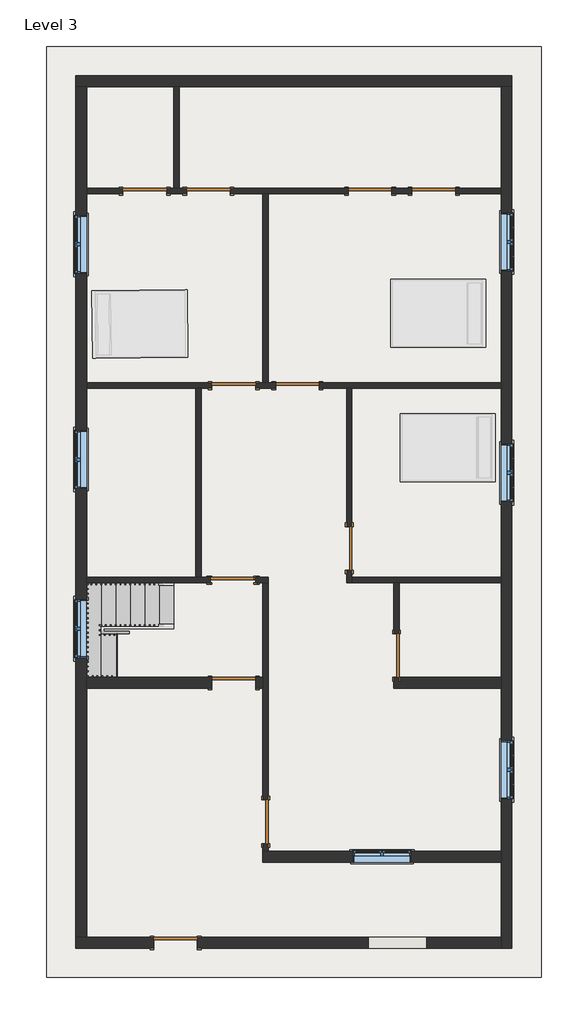
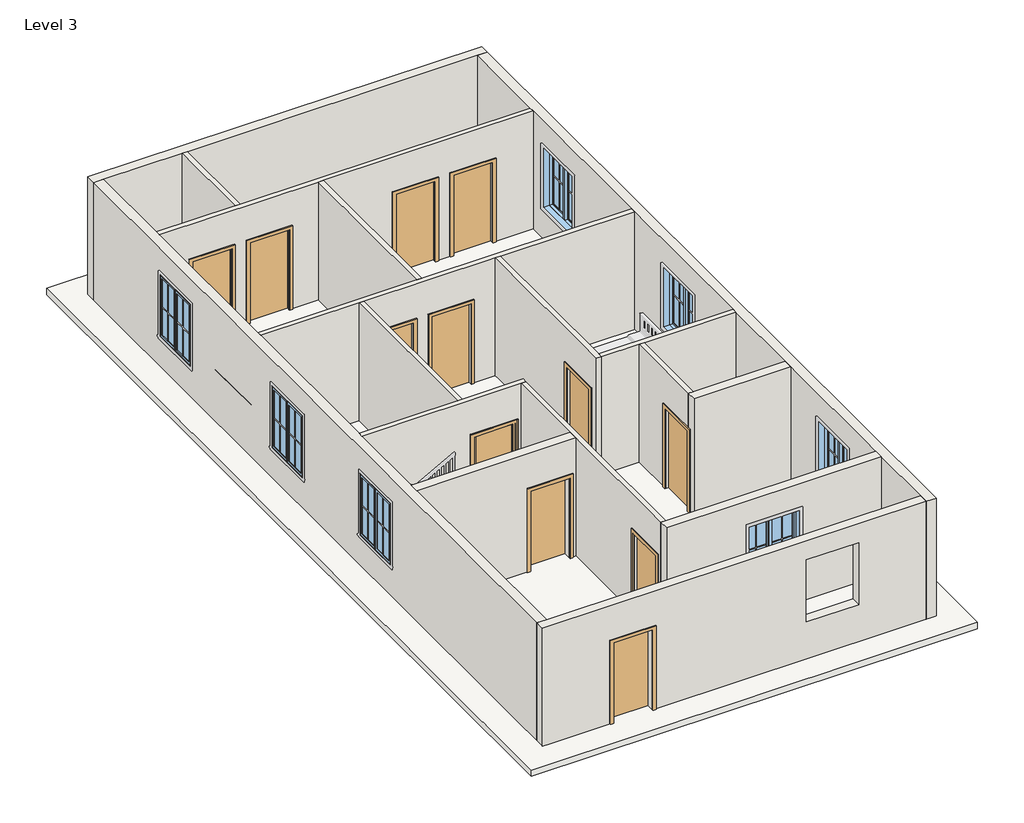
# One storey, part 1 of 2: 17 walls, 13 doors, 7 windows, 1 roof, 1 stair flight.
"""IFC4 building model written with IfcOpenShell, lengths in millimetres."""

from ifc_helpers import new_model, si_unit, frame, origin, place, context, project, spatial, polyline, outline, extrude, faceted_brep, transform, mapped, element, save
from components import door_e5f9f3c4, door_305aa2a5, door_0ca8825f, stair_flight_2df44192, window_8377141f

model = new_model("IFC4")

# Units and contexts
model_context = context("Model", 3, world=origin())
ifc_project = project(units=[si_unit("LENGTHUNIT", "METRE", prefix="MILLI")], contexts=[model_context])

# Site, building, storey
site = spatial("IfcSite", under=ifc_project)
building = spatial("IfcBuilding", under=site)
storey = spatial("IfcBuildingStorey", under=building, Name="Level 3", Elevation=6096.0)

# Doors
placement = place(None, origin())
door_shape = door_e5f9f3c4(model_context)
element("IfcDoor", 1, ObjectType="Single-Flush : 36\" x 84\"", at=placement, inside=storey, context=model_context, shape_type="MappedRepresentation", body=[
    mapped(door_shape, transform((7442.2, 11550.65, 6096.0), x_axis=(1.0, 0.0, 0.0), y_axis=(0.0, 1.0, 0.0), z_axis=(0.0, 0.0, 1.0))),
])
element("IfcDoor", 2, ObjectType="Single-Flush : 36\" x 84\"", at=placement, inside=storey, context=model_context, shape_type="MappedRepresentation", body=[
    mapped(door_shape, transform((2717.8, 11550.65, 6096.0), x_axis=(1.0, 0.0, 0.0), y_axis=(0.0, 1.0, 0.0), z_axis=(0.0, 0.0, 1.0))),
])
element("IfcDoor", 3, ObjectType="Single-Flush : 36\" x 84\"", at=placement, inside=storey, context=model_context, shape_type="MappedRepresentation", body=[
    mapped(door_shape, transform((4584.7, 7473.95, 6096.0), x_axis=(1.0, 0.0, 0.0), y_axis=(0.0, 1.0, 0.0), z_axis=(0.0, 0.0, 1.0))),
])
element("IfcDoor", 4, ObjectType="Single-Flush : 36\" x 84\"", at=placement, inside=storey, context=model_context, shape_type="MappedRepresentation", body=[
    mapped(door_shape, transform((4546.6, 3397.25, 6096.0), x_axis=(1.0, 0.0, 0.0), y_axis=(0.0, 1.0, 0.0), z_axis=(0.0, 0.0, 1.0))),
])
element("IfcDoor", 5, ObjectType="Single-Flush : 36\" x 84\"", at=placement, inside=storey, context=model_context, shape_type="MappedRepresentation", body=[
    mapped(door_shape, transform((4584.7, 3397.25, 6096.0), x_axis=(1.0, 0.0, 0.0), y_axis=(0.0, 1.0, 0.0), z_axis=(0.0, 0.0, 1.0))),
])
element("IfcDoor", 6, ObjectType="Single-Flush : 36\" x 84\"", at=placement, inside=storey, context=model_context, shape_type="MappedRepresentation", body=[
    mapped(door_shape, transform((7004.05, 4064.0, 6096.0), x_axis=(0.0, -1.0, 0.0), y_axis=(1.0, 0.0, 0.0), z_axis=(0.0, 0.0, 1.0))),
])
element("IfcDoor", 7, ObjectType="Single-Flush : 36\" x 84\"", at=placement, inside=storey, context=model_context, shape_type="MappedRepresentation", body=[
    mapped(door_shape, transform((5251.45, -1663.7, 6096.0), x_axis=(0.0, -1.0, 0.0), y_axis=(1.0, 0.0, 0.0), z_axis=(0.0, 0.0, 1.0))),
])
door_2_shape = door_305aa2a5(model_context)
element("IfcDoor", 8, ObjectType="Single-Flush : 36\" x 84\"", at=placement, inside=storey, context=model_context, shape_type="MappedRepresentation", body=[
    mapped(door_2_shape, transform((4051.3, 11550.65, 6096.0), x_axis=(-1.0, 0.0, 0.0), y_axis=(0.0, -1.0, 0.0), z_axis=(0.0, 0.0, 1.0))),
])
element("IfcDoor", 9, ObjectType="Single-Flush : 36\" x 84\"", at=placement, inside=storey, context=model_context, shape_type="MappedRepresentation", body=[
    mapped(door_2_shape, transform((5918.2, 7473.95, 6096.0), x_axis=(-1.0, 0.0, 0.0), y_axis=(0.0, -1.0, 0.0), z_axis=(0.0, 0.0, 1.0))),
])
element("IfcDoor", 10, ObjectType="Single-Flush : 36\" x 84\"", at=placement, inside=storey, context=model_context, shape_type="MappedRepresentation", body=[
    mapped(door_2_shape, transform((7994.65, 1816.1, 6096.0), x_axis=(0.0, 1.0, 0.0), y_axis=(-1.0, 0.0, 0.0), z_axis=(0.0, 0.0, 1.0))),
])
element("IfcDoor", 11, ObjectType="Single-Flush : 36\" x 84\"", at=placement, inside=storey, context=model_context, shape_type="MappedRepresentation", body=[
    mapped(door_2_shape, transform((8775.7, 11550.65, 6096.0), x_axis=(-1.0, 0.0, 0.0), y_axis=(0.0, -1.0, 0.0), z_axis=(0.0, 0.0, 1.0))),
])
door_3_shape = door_0ca8825f(model_context)
element("IfcDoor", 12, ObjectType="Single-Flush : 36\" x 84\"", at=placement, inside=storey, context=model_context, shape_type="MappedRepresentation", body=[
    mapped(door_3_shape, transform((4584.7, 1244.6, 6096.0), x_axis=(1.0, 0.0, 0.0), y_axis=(0.0, 1.0, 0.0), z_axis=(0.0, 0.0, 1.0))),
])
element("IfcDoor", 13, ObjectType="Single-Flush : 36\" x 84\"", at=placement, inside=storey, context=model_context, shape_type="MappedRepresentation", body=[
    mapped(door_3_shape, transform((3365.5, -4203.7, 6096.0), x_axis=(1.0, 0.0, 0.0), y_axis=(0.0, 1.0, 0.0), z_axis=(0.0, 0.0, 1.0))),
])

# Roof
element("IfcRoof", 14, ObjectType="Generic - 12\"", at=placement, inside=storey, context=model_context, shape_type="SweptSolid", body=[
    extrude(outline(polyline([(660.4, 14579.6), (11023.6, 14579.6), (11023.6, -4927.6), (660.4, -4927.6), (660.4, 14579.6)])), frame((0.0, 0.0, 6096.0), z_axis=(0.0, 0.0, 1.0), x_axis=(1.0, 0.0, 0.0)), (0.0, 0.0, 1.0), 152.4),
])

# Stair flight
stair_flight_shape = stair_flight_2df44192(model_context)
element("IfcStairFlight", 15, ObjectType="2\" Tread 1\" Nosing 1/4\" Riser", at=placement, inside=storey, context=model_context, shape_type="MappedRepresentation", body=[
    mapped(stair_flight_shape, transform((0.0, 0.0, 0.0), x_axis=(1.0, 0.0, 0.0), y_axis=(0.0, 1.0, 0.0), z_axis=(0.0, 0.0, 1.0))),
])

# Walls
element("IfcWall", 16, ObjectType="Generic - 5\"", at=placement, inside=storey, context=model_context, shape_type="SweptSolid", body=[
    extrude(outline(polyline([(3327.4, 11607.8), (3327.4, 13741.4), (3441.7, 13741.4), (3441.7, 11607.8), (3327.4, 11607.8)])), frame((0.0, 0.0, 6096.0), z_axis=(0.0, 0.0, 1.0), x_axis=(1.0, 0.0, 0.0)), (0.0, 0.0, 1.0), 3048.0),
])
element("IfcWall", 17, ObjectType="Generic - 5\"", at=placement, inside=storey, context=model_context, shape_type="Brep", body=[
    faceted_brep([(7899.4, 11493.5, 6096.0), (8318.5, 11493.5, 6096.0), (8318.5, 11493.5, 8229.6), (9232.9, 11493.5, 8229.6), (9232.9, 11493.5, 6096.0), (10185.4, 11493.5, 6096.0), (10185.4, 11493.5, 9144.0), (5308.6, 11493.5, 9144.0), (5194.3, 11493.5, 9144.0), (1498.6, 11493.5, 9144.0), (1498.6, 11493.5, 6096.0), (2260.6, 11493.5, 6096.0), (2260.6, 11493.5, 8229.6), (3175.0, 11493.5, 8229.6), (3175.0, 11493.5, 6096.0), (3594.1, 11493.5, 6096.0), (3594.1, 11493.5, 8229.6), (4508.5, 11493.5, 8229.6), (4508.5, 11493.5, 6096.0), (5194.3, 11493.5, 6096.0), (5308.6, 11493.5, 6096.0), (6985.0, 11493.5, 6096.0), (6985.0, 11493.5, 8229.6), (7899.4, 11493.5, 8229.6), (8318.5, 11607.8, 8229.6), (8318.5, 11607.8, 6096.0), (7899.4, 11607.8, 6096.0), (7899.4, 11607.8, 8229.6), (6985.0, 11607.8, 8229.6), (6985.0, 11607.8, 6096.0), (4508.5, 11607.8, 6096.0), (4508.5, 11607.8, 8229.6), (3594.1, 11607.8, 8229.6), (3594.1, 11607.8, 6096.0), (3441.7, 11607.8, 6096.0), (3327.4, 11607.8, 6096.0), (3175.0, 11607.8, 6096.0), (3175.0, 11607.8, 8229.6), (2260.6, 11607.8, 8229.6), (2260.6, 11607.8, 6096.0), (1498.6, 11607.8, 6096.0), (1498.6, 11607.8, 9144.0), (3327.4, 11607.8, 9144.0), (3441.7, 11607.8, 9144.0), (10185.4, 11607.8, 9144.0), (10185.4, 11607.8, 6096.0), (9232.9, 11607.8, 6096.0), (9232.9, 11607.8, 8229.6)], [[[0, 1, 2, 3, 4, 5, 6, 7, 8, 9, 10, 11, 12, 13, 14, 15, 16, 17, 18, 19, 20, 21, 22, 23]], [[24, 25, 26, 27, 28, 29, 30, 31, 32, 33, 34, 35, 36, 37, 38, 39, 40, 41, 42, 43, 44, 45, 46, 47]], [[11, 10, 40, 39]], [[30, 29, 21, 20, 19, 18]], [[36, 35, 34, 33, 15, 14]], [[46, 45, 5, 4]], [[26, 25, 1, 0]], [[9, 8, 7, 6, 44, 43, 42, 41]], [[6, 5, 45, 44]], [[10, 9, 41, 40]], [[27, 26, 0, 23]], [[28, 27, 23, 22]], [[29, 28, 22, 21]], [[37, 36, 14, 13]], [[38, 37, 13, 12]], [[39, 38, 12, 11]], [[16, 15, 33, 32]], [[17, 16, 32, 31]], [[18, 17, 31, 30]], [[2, 1, 25, 24]], [[3, 2, 24, 47]], [[4, 3, 47, 46]]]),
])
element("IfcWall", 18, ObjectType="Generic - 5\"", at=placement, inside=storey, context=model_context, shape_type="Brep", body=[
    faceted_brep([(5041.9, 7416.8, 8229.6), (5041.9, 7416.8, 6096.0), (5461.0, 7416.8, 6096.0), (5461.0, 7416.8, 8229.6), (6375.4, 7416.8, 8229.6), (6375.4, 7416.8, 6096.0), (6946.9, 7416.8, 6096.0), (7061.2, 7416.8, 6096.0), (10185.4, 7416.8, 6096.0), (10185.4, 7416.8, 9144.0), (7061.2, 7416.8, 9144.0), (6946.9, 7416.8, 9144.0), (3898.9, 7416.8, 9144.0), (3784.6, 7416.8, 9144.0), (1498.6, 7416.8, 9144.0), (1498.6, 7416.8, 6096.0), (3784.6, 7416.8, 6096.0), (3898.9, 7416.8, 6096.0), (4127.5, 7416.8, 6096.0), (4127.5, 7416.8, 8229.6), (5461.0, 7531.1, 6096.0), (5308.6, 7531.1, 6096.0), (5194.3, 7531.1, 6096.0), (5041.9, 7531.1, 6096.0), (5041.9, 7531.1, 8229.6), (4127.5, 7531.1, 8229.6), (4127.5, 7531.1, 6096.0), (1498.6, 7531.1, 6096.0), (1498.6, 7531.1, 9144.0), (5194.3, 7531.1, 9144.0), (5308.6, 7531.1, 9144.0), (10185.4, 7531.1, 9144.0), (10185.4, 7531.1, 6096.0), (6375.4, 7531.1, 6096.0), (6375.4, 7531.1, 8229.6), (5461.0, 7531.1, 8229.6)], [[[0, 1, 2, 3, 4, 5, 6, 7, 8, 9, 10, 11, 12, 13, 14, 15, 16, 17, 18, 19]], [[20, 21, 22, 23, 24, 25, 26, 27, 28, 29, 30, 31, 32, 33, 34, 35]], [[33, 32, 8, 7, 6, 5]], [[2, 1, 23, 22, 21, 20]], [[18, 17, 16, 15, 27, 26]], [[14, 13, 12, 11, 10, 9, 31, 30, 29, 28]], [[9, 8, 32, 31]], [[15, 14, 28, 27]], [[3, 2, 20, 35]], [[4, 3, 35, 34]], [[5, 4, 34, 33]], [[24, 23, 1, 0]], [[25, 24, 0, 19]], [[26, 25, 19, 18]]]),
])
element("IfcWall", 19, ObjectType="Generic - 5\"", at=placement, inside=storey, context=model_context, shape_type="SweptSolid", body=[
    extrude(outline(polyline([(5194.3, 7531.1), (5194.3, 11493.5), (5308.6, 11493.5), (5308.6, 7531.1), (5194.3, 7531.1)])), frame((0.0, 0.0, 6096.0), z_axis=(0.0, 0.0, 1.0), x_axis=(1.0, 0.0, 0.0)), (0.0, 0.0, 1.0), 3048.0),
])
element("IfcWall", 20, ObjectType="Generic - 5\"", at=placement, inside=storey, context=model_context, shape_type="SweptSolid", body=[
    extrude(outline(polyline([(3784.6, 3454.4), (3784.6, 7416.8), (3898.9, 7416.8), (3898.9, 3454.4), (3784.6, 3454.4)])), frame((0.0, 0.0, 6096.0), z_axis=(0.0, 0.0, 1.0), x_axis=(1.0, 0.0, 0.0)), (0.0, 0.0, 1.0), 3048.0),
])
element("IfcWall", 21, ObjectType="Generic - 5\"", at=placement, inside=storey, context=model_context, shape_type="Brep", body=[
    faceted_brep([(5308.6, 3340.1, 9144.0), (5194.3, 3340.1, 9144.0), (1498.6, 3340.1, 9144.0), (1498.6, 3340.1, 6096.0), (4089.4, 3340.1, 6096.0), (4089.4, 3340.1, 8229.6), (5041.9, 3340.1, 8229.6), (5041.9, 3340.1, 6096.0), (5194.3, 3340.1, 6096.0), (5308.6, 3340.1, 6096.0), (1498.6, 3454.4, 9144.0), (3784.6, 3454.4, 9144.0), (3898.9, 3454.4, 9144.0), (5308.6, 3454.4, 9144.0), (5308.6, 3454.4, 6096.0), (5041.9, 3454.4, 6096.0), (5041.9, 3454.4, 8229.6), (4089.4, 3454.4, 8229.6), (4089.4, 3454.4, 6096.0), (3898.9, 3454.4, 6096.0), (3784.6, 3454.4, 6096.0), (1498.6, 3454.4, 6096.0)], [[[0, 1, 2, 3, 4, 5, 6, 7, 8, 9]], [[10, 11, 12, 13, 14, 15, 16, 17, 18, 19, 20, 21]], [[3, 21, 20, 19, 18, 4]], [[14, 9, 8, 7, 15]], [[2, 1, 0, 13, 12, 11, 10]], [[3, 2, 10, 21]], [[0, 9, 14, 13]], [[5, 17, 16, 6]], [[18, 17, 5, 4]], [[6, 16, 15, 7]]]),
])
element("IfcWall", 22, ObjectType="Generic - 5\"", at=placement, inside=storey, context=model_context, shape_type="Brep", body=[
    faceted_brep([(5194.3, -2120.9, 8229.6), (5194.3, -2120.9, 6096.0), (5194.3, -2286.0, 6096.0), (5194.3, -2286.0, 9144.0), (5194.3, 1130.3, 9144.0), (5194.3, 1358.9, 9144.0), (5194.3, 3340.1, 9144.0), (5194.3, 3340.1, 6096.0), (5194.3, 1358.9, 6096.0), (5194.3, 1130.3, 6096.0), (5194.3, -1206.5, 6096.0), (5194.3, -1206.5, 8229.6), (5308.6, -2286.0, 6096.0), (5308.6, -2120.9, 6096.0), (5308.6, -2120.9, 8229.6), (5308.6, -1206.5, 8229.6), (5308.6, -1206.5, 6096.0), (5308.6, 3340.1, 6096.0), (5308.6, 3340.1, 9144.0), (5308.6, -2286.0, 9144.0)], [[[0, 1, 2, 3, 4, 5, 6, 7, 8, 9, 10, 11]], [[12, 13, 14, 15, 16, 17, 18, 19]], [[2, 1, 13, 12]], [[10, 9, 8, 7, 17, 16]], [[6, 5, 4, 3, 19, 18]], [[7, 6, 18, 17]], [[3, 2, 12, 19]], [[14, 13, 1, 0]], [[15, 14, 0, 11]], [[16, 15, 11, 10]]]),
])
element("IfcWall", 23, ObjectType="Generic - 5\"", at=placement, inside=storey, context=model_context, shape_type="Brep", body=[
    faceted_brep([(6946.9, 3606.8, 8229.6), (6946.9, 3606.8, 6096.0), (6946.9, 3340.1, 6096.0), (6946.9, 3340.1, 9144.0), (6946.9, 7416.8, 9144.0), (6946.9, 7416.8, 6096.0), (6946.9, 4521.2, 6096.0), (6946.9, 4521.2, 8229.6), (7061.2, 3340.1, 6096.0), (7061.2, 3454.4, 6096.0), (7061.2, 3606.8, 6096.0), (7061.2, 3606.8, 8229.6), (7061.2, 4521.2, 8229.6), (7061.2, 4521.2, 6096.0), (7061.2, 7416.8, 6096.0), (7061.2, 7416.8, 9144.0), (7061.2, 3454.4, 9144.0), (7061.2, 3340.1, 9144.0)], [[[0, 1, 2, 3, 4, 5, 6, 7]], [[8, 9, 10, 11, 12, 13, 14, 15, 16, 17]], [[6, 5, 14, 13]], [[2, 1, 10, 9, 8]], [[4, 3, 17, 16, 15]], [[5, 4, 15, 14]], [[3, 2, 8, 17]], [[11, 10, 1, 0]], [[12, 11, 0, 7]], [[13, 12, 7, 6]]]),
])
element("IfcWall", 24, ObjectType="Generic - 5\"", at=placement, inside=storey, context=model_context, shape_type="SweptSolid", body=[
    extrude(outline(polyline([(1358.9, 9144.0), (3340.1, 9144.0), (3340.1, 6096.0), (2273.3, 6096.0), (2273.3, 8229.6), (1358.9, 8229.6), (1358.9, 9144.0)])), frame((7937.5, 0.0, 0.0), z_axis=(1.0, 0.0, 0.0), x_axis=(0.0, 1.0, 0.0)), (0.0, 0.0, 1.0), 114.3),
])
element("IfcWall", 25, ObjectType="Generic - 5\"", at=placement, inside=storey, context=model_context, shape_type="Brep", body=[
    faceted_brep([(7061.2, 3340.1, 6096.0), (7937.5, 3340.1, 6096.0), (8051.8, 3340.1, 6096.0), (10185.4, 3340.1, 6096.0), (10185.4, 3340.1, 9144.0), (8051.8, 3340.1, 9144.0), (7937.5, 3340.1, 9144.0), (7061.2, 3340.1, 9144.0), (7061.2, 3454.4, 6096.0), (7061.2, 3454.4, 9144.0), (10185.4, 3454.4, 9144.0), (10185.4, 3454.4, 6096.0)], [[[0, 1, 2, 3, 4, 5, 6, 7]], [[8, 9, 10, 11]], [[3, 2, 1, 0, 8, 11]], [[7, 6, 5, 4, 10, 9]], [[0, 7, 9, 8]], [[4, 3, 11, 10]]]),
])
element("IfcWall", 26, ObjectType="Generic - 8\"", at=placement, inside=storey, context=model_context, shape_type="Brep", body=[
    faceted_brep([(1270.0, 13741.4, 6096.0), (1498.6, 13741.4, 6096.0), (3327.4, 13741.4, 6096.0), (3441.7, 13741.4, 6096.0), (10185.4, 13741.4, 6096.0), (10414.0, 13741.4, 6096.0), (10414.0, 13741.4, 9144.0), (10185.4, 13741.4, 9144.0), (3441.7, 13741.4, 9144.0), (3327.4, 13741.4, 9144.0), (1498.6, 13741.4, 9144.0), (1270.0, 13741.4, 9144.0), (1270.0, 13970.0, 6096.0), (1270.0, 13970.0, 9144.0), (10414.0, 13970.0, 9144.0), (10414.0, 13970.0, 6096.0)], [[[0, 1, 2, 3, 4, 5, 6, 7, 8, 9, 10, 11]], [[12, 13, 14, 15]], [[5, 4, 3, 2, 1, 0, 12, 15]], [[11, 10, 9, 8, 7, 6, 14, 13]], [[6, 5, 15, 14]], [[0, 11, 13, 12]]]),
])
element("IfcWall", 27, ObjectType="Generic - 8\"", at=placement, inside=storey, context=model_context, shape_type="Brep", body=[
    faceted_brep([(10185.4, 13741.4, 6096.0), (10185.4, 11607.8, 6096.0), (10185.4, 11493.5, 6096.0), (10185.4, 7531.1, 6096.0), (10185.4, 7416.8, 6096.0), (10185.4, 3454.4, 6096.0), (10185.4, 3340.1, 6096.0), (10185.4, 1358.9, 6096.0), (10185.4, 1130.3, 6096.0), (10185.4, -2286.0, 6096.0), (10185.4, -2514.6, 6096.0), (10185.4, -4089.4, 6096.0), (10185.4, -4318.0, 6096.0), (10185.4, -4318.0, 9144.0), (10185.4, -4089.4, 9144.0), (10185.4, -2514.6, 9144.0), (10185.4, -2286.0, 9144.0), (10185.4, 1130.3, 9144.0), (10185.4, 1358.9, 9144.0), (10185.4, 3340.1, 9144.0), (10185.4, 3454.4, 9144.0), (10185.4, 7416.8, 9144.0), (10185.4, 7531.1, 9144.0), (10185.4, 11493.5, 9144.0), (10185.4, 11607.8, 9144.0), (10185.4, 13741.4, 9144.0), (10185.4, 9874.25, 8534.4), (10185.4, 9874.25, 7010.4), (10185.4, 11093.45, 7010.4), (10185.4, 11093.45, 8534.4), (10185.4, 5035.55, 8534.4), (10185.4, 5035.55, 7010.4), (10185.4, 6254.75, 7010.4), (10185.4, 6254.75, 8534.4), (10185.4, -1187.45, 8534.4), (10185.4, -1187.45, 7010.4), (10185.4, 31.75, 7010.4), (10185.4, 31.75, 8534.4), (10414.0, 13741.4, 6096.0), (10414.0, 13741.4, 9144.0), (10414.0, -4318.0, 9144.0), (10414.0, -4318.0, 6096.0), (10414.0, 9874.25, 8534.4), (10414.0, 11093.45, 8534.4), (10414.0, 11093.45, 7010.4), (10414.0, 9874.25, 7010.4), (10414.0, 5035.55, 8534.4), (10414.0, 6254.75, 8534.4), (10414.0, 6254.75, 7010.4), (10414.0, 5035.55, 7010.4), (10414.0, -1187.45, 8534.4), (10414.0, 31.75, 8534.4), (10414.0, 31.75, 7010.4), (10414.0, -1187.45, 7010.4)], [[[0, 1, 2, 3, 4, 5, 6, 7, 8, 9, 10, 11, 12, 13, 14, 15, 16, 17, 18, 19, 20, 21, 22, 23, 24, 25], [26, 27, 28, 29], [30, 31, 32, 33], [34, 35, 36, 37]], [[38, 39, 40, 41], [42, 43, 44, 45], [46, 47, 48, 49], [50, 51, 52, 53]], [[12, 11, 10, 9, 8, 7, 6, 5, 4, 3, 2, 1, 0, 38, 41]], [[25, 24, 23, 22, 21, 20, 19, 18, 17, 16, 15, 14, 13, 40, 39]], [[0, 25, 39, 38]], [[13, 12, 41, 40]], [[27, 26, 42, 45]], [[28, 27, 45, 44]], [[29, 28, 44, 43]], [[26, 29, 43, 42]], [[31, 30, 46, 49]], [[32, 31, 49, 48]], [[33, 32, 48, 47]], [[30, 33, 47, 46]], [[35, 34, 50, 53]], [[36, 35, 53, 52]], [[37, 36, 52, 51]], [[34, 37, 51, 50]]]),
])
element("IfcWall", 28, ObjectType="Generic - 8\"", at=placement, inside=storey, context=model_context, shape_type="Brep", body=[
    faceted_brep([(10185.4, -4089.4, 6096.0), (3822.7, -4089.4, 6096.0), (3822.7, -4089.4, 8229.6), (2908.3, -4089.4, 8229.6), (2908.3, -4089.4, 6096.0), (1498.6, -4089.4, 6096.0), (1270.0, -4089.4, 6096.0), (1270.0, -4089.4, 9144.0), (1498.6, -4089.4, 9144.0), (10185.4, -4089.4, 9144.0), (7404.1, -4089.4, 8679.7309921), (7404.1, -4089.4, 7155.7309921), (8623.3, -4089.4, 7155.7309921), (8623.3, -4089.4, 8679.7309921), (3822.7, -4318.0, 8229.6), (3822.7, -4318.0, 6096.0), (10185.4, -4318.0, 6096.0), (10185.4, -4318.0, 9144.0), (1270.0, -4318.0, 9144.0), (1270.0, -4318.0, 6096.0), (2908.3, -4318.0, 6096.0), (2908.3, -4318.0, 8229.6), (7404.1, -4318.0, 8679.7309921), (8623.3, -4318.0, 8679.7309921), (8623.3, -4318.0, 7155.7309921), (7404.1, -4318.0, 7155.7309921)], [[[0, 1, 2, 3, 4, 5, 6, 7, 8, 9], [10, 11, 12, 13]], [[14, 15, 16, 17, 18, 19, 20, 21], [22, 23, 24, 25]], [[20, 19, 6, 5, 4]], [[16, 15, 1, 0]], [[9, 8, 7, 18, 17]], [[0, 9, 17, 16]], [[7, 6, 19, 18]], [[2, 1, 15, 14]], [[3, 2, 14, 21]], [[4, 3, 21, 20]], [[11, 10, 22, 25]], [[12, 11, 25, 24]], [[13, 12, 24, 23]], [[10, 13, 23, 22]]]),
])
element("IfcWall", 29, ObjectType="Generic - 8\"", at=placement, inside=storey, context=model_context, shape_type="Brep", body=[
    faceted_brep([(1498.6, -4089.4, 6096.0), (1498.6, 1130.3, 6096.0), (1498.6, 1358.9, 6096.0), (1498.6, 3340.1, 6096.0), (1498.6, 3454.4, 6096.0), (1498.6, 7416.8, 6096.0), (1498.6, 7531.1, 6096.0), (1498.6, 11493.5, 6096.0), (1498.6, 11607.8, 6096.0), (1498.6, 13741.4, 6096.0), (1498.6, 13741.4, 9144.0), (1498.6, 11607.8, 9144.0), (1498.6, 11493.5, 9144.0), (1498.6, 7531.1, 9144.0), (1498.6, 7416.8, 9144.0), (1498.6, 3454.4, 9144.0), (1498.6, 3340.1, 9144.0), (1498.6, 1358.9, 9144.0), (1498.6, 1130.3, 9144.0), (1498.6, -4089.4, 9144.0), (1498.6, 6534.15, 8534.4), (1498.6, 6534.15, 7010.4), (1498.6, 5314.95, 7010.4), (1498.6, 5314.95, 8534.4), (1498.6, 11042.65, 8534.4), (1498.6, 11042.65, 7010.4), (1498.6, 9823.45, 7010.4), (1498.6, 9823.45, 8534.4), (1498.6, 2990.85, 8534.4), (1498.6, 2990.85, 7010.4), (1498.6, 1771.65, 7010.4), (1498.6, 1771.65, 8534.4), (1270.0, -4089.4, 6096.0), (1270.0, -4089.4, 9144.0), (1270.0, 13741.4, 9144.0), (1270.0, 13741.4, 6096.0), (1270.0, 6534.15, 8534.4), (1270.0, 5314.95, 8534.4), (1270.0, 5314.95, 7010.4), (1270.0, 6534.15, 7010.4), (1270.0, 11042.65, 8534.4), (1270.0, 9823.45, 8534.4), (1270.0, 9823.45, 7010.4), (1270.0, 11042.65, 7010.4), (1270.0, 2990.85, 8534.4), (1270.0, 1771.65, 8534.4), (1270.0, 1771.65, 7010.4), (1270.0, 2990.85, 7010.4)], [[[0, 1, 2, 3, 4, 5, 6, 7, 8, 9, 10, 11, 12, 13, 14, 15, 16, 17, 18, 19], [20, 21, 22, 23], [24, 25, 26, 27], [28, 29, 30, 31]], [[32, 33, 34, 35], [36, 37, 38, 39], [40, 41, 42, 43], [44, 45, 46, 47]], [[9, 8, 7, 6, 5, 4, 3, 2, 1, 0, 32, 35]], [[19, 18, 17, 16, 15, 14, 13, 12, 11, 10, 34, 33]], [[10, 9, 35, 34]], [[0, 19, 33, 32]], [[21, 20, 36, 39]], [[22, 21, 39, 38]], [[23, 22, 38, 37]], [[20, 23, 37, 36]], [[25, 24, 40, 43]], [[26, 25, 43, 42]], [[27, 26, 42, 41]], [[24, 27, 41, 40]], [[29, 28, 44, 47]], [[30, 29, 47, 46]], [[31, 30, 46, 45]], [[28, 31, 45, 44]]]),
])
element("IfcWall", 30, ObjectType="Generic - 8\"", at=placement, inside=storey, context=model_context, shape_type="SweptSolid", body=[
    extrude(outline(polyline([(8229.6, 5041.9), (6096.0, 5041.9), (6096.0, 5194.3), (9144.0, 5194.3), (9144.0, 1498.6), (6096.0, 1498.6), (6096.0, 4127.5), (8229.6, 4127.5), (8229.6, 5041.9)])), frame((0.0, 1130.3, 0.0), z_axis=(0.0, 1.0, 0.0), x_axis=(0.0, 0.0, 1.0)), (0.0, 0.0, 1.0), 228.6),
])
element("IfcWall", 31, ObjectType="Generic - 8\"", at=placement, inside=storey, context=model_context, shape_type="Brep", body=[
    faceted_brep([(5194.3, -2514.6, 6096.0), (10185.4, -2514.6, 6096.0), (10185.4, -2514.6, 9144.0), (5194.3, -2514.6, 9144.0), (8299.45, -2514.6, 8534.4), (8299.45, -2514.6, 7010.4), (7080.25, -2514.6, 7010.4), (7080.25, -2514.6, 8534.4), (5194.3, -2286.0, 6096.0), (5194.3, -2286.0, 9144.0), (5308.6, -2286.0, 9144.0), (10185.4, -2286.0, 9144.0), (10185.4, -2286.0, 6096.0), (5308.6, -2286.0, 6096.0), (8299.45, -2286.0, 8534.4), (7080.25, -2286.0, 8534.4), (7080.25, -2286.0, 7010.4), (8299.45, -2286.0, 7010.4)], [[[0, 1, 2, 3], [4, 5, 6, 7]], [[8, 9, 10, 11, 12, 13], [14, 15, 16, 17]], [[1, 0, 8, 13, 12]], [[3, 2, 11, 10, 9]], [[0, 3, 9, 8]], [[2, 1, 12, 11]], [[5, 4, 14, 17]], [[6, 5, 17, 16]], [[7, 6, 16, 15]], [[4, 7, 15, 14]]]),
])
element("IfcWall", 32, ObjectType="Generic - 8\"", at=placement, inside=storey, context=model_context, shape_type="Brep", body=[
    faceted_brep([(7937.5, 1130.3, 6096.0), (10185.4, 1130.3, 6096.0), (10185.4, 1130.3, 9144.0), (7937.5, 1130.3, 9144.0), (7937.5, 1358.9, 6096.0), (7937.5, 1358.9, 8229.6), (7937.5, 1358.9, 9144.0), (8051.8, 1358.9, 9144.0), (10185.4, 1358.9, 9144.0), (10185.4, 1358.9, 6096.0)], [[[0, 1, 2, 3]], [[4, 5, 6, 7, 8, 9]], [[1, 0, 4, 9]], [[3, 2, 8, 7, 6]], [[0, 3, 6, 5, 4]], [[2, 1, 9, 8]]]),
])

# Windows
window_shape = window_8377141f(model_context)
element("IfcWindow", 33, ObjectType="Window-Casement-Double : 48\" x 60\"", at=placement, inside=storey, context=model_context, shape_type="MappedRepresentation", body=[
    mapped(window_shape, transform((1384.3, 5924.55, 6096.0), x_axis=(0.0, 1.0, 0.0), y_axis=(-1.0, 0.0, 0.0), z_axis=(0.0, 0.0, 1.0))),
])
element("IfcWindow", 34, ObjectType="Window-Casement-Double : 48\" x 60\"", at=placement, inside=storey, context=model_context, shape_type="MappedRepresentation", body=[
    mapped(window_shape, transform((1384.3, 10433.05, 6096.0), x_axis=(0.0, 1.0, 0.0), y_axis=(-1.0, 0.0, 0.0), z_axis=(0.0, 0.0, 1.0))),
])
element("IfcWindow", 35, ObjectType="Window-Casement-Double : 48\" x 60\"", at=placement, inside=storey, context=model_context, shape_type="MappedRepresentation", body=[
    mapped(window_shape, transform((10299.7, 10483.85, 6096.0), x_axis=(0.0, -1.0, 0.0), y_axis=(1.0, 0.0, 0.0), z_axis=(0.0, 0.0, 1.0))),
])
element("IfcWindow", 36, ObjectType="Window-Casement-Double : 48\" x 60\"", at=placement, inside=storey, context=model_context, shape_type="MappedRepresentation", body=[
    mapped(window_shape, transform((10299.7, 5645.15, 6096.0), x_axis=(0.0, -1.0, 0.0), y_axis=(1.0, 0.0, 0.0), z_axis=(0.0, 0.0, 1.0))),
])
element("IfcWindow", 37, ObjectType="Window-Casement-Double : 48\" x 60\"", at=placement, inside=storey, context=model_context, shape_type="MappedRepresentation", body=[
    mapped(window_shape, transform((10299.7, -577.85, 6096.0), x_axis=(0.0, -1.0, 0.0), y_axis=(1.0, 0.0, 0.0), z_axis=(0.0, 0.0, 1.0))),
])
element("IfcWindow", 38, ObjectType="Window-Casement-Double : 48\" x 60\"", at=placement, inside=storey, context=model_context, shape_type="MappedRepresentation", body=[
    mapped(window_shape, transform((7689.85, -2400.3, 6096.0), x_axis=(1.0, 0.0, 0.0), y_axis=(0.0, 1.0, 0.0), z_axis=(0.0, 0.0, 1.0))),
])
element("IfcWindow", 39, ObjectType="Window-Casement-Double : 48\" x 60\"", at=placement, inside=storey, context=model_context, shape_type="MappedRepresentation", body=[
    mapped(window_shape, transform((1384.3, 2381.25, 6096.0), x_axis=(0.0, 1.0, 0.0), y_axis=(-1.0, 0.0, 0.0), z_axis=(0.0, 0.0, 1.0))),
])

save(model, "model.ifc")

# Revit data of these elements
# Type "Single-Flush : 36\" x 84\""
#   Type Mark = "1"
#   Construction Type Id = "MDOOR"
#   Assembly Code = "C1020"
#   Analytic Construction = "Metal"
#   Thickness = 0' - 2"
#   Heat Transfer Coefficient (U) = 0.651978 BTU/(h·ft²·°F)
#   Height = 7' - 0"
#   Trim Projection Ext = 0' - 1"
#   Trim Projection Int = 0' - 1"
#   Trim Width = 0' - 3"
#   Width = 3' - 0"
#   Define Thermal Properties by = 1
#   Define Thermal Properties by = 1
#   Door Material = Door - Panel
#   Frame Material = Door - Frame
#   Visual Light Transmittance = 0
#   Solar Heat Gain Coefficient = 0
#   Function = (empty or 0)
#   Wall Closure = (empty or 0)
# Type "Generic - 12\""
#   Assembly Code = "B1020"
#   Layers, outside or top first: 0' - 6" no material (function 1)
# Type "Generic - 5\""
#   Assembly Code = "B2010"
#   Layers, outside or top first: 0' - 4 1/2" no material (function 1)
# Type "Generic - 8\""
#   Assembly Code = "B2010"
# Type "Window-Casement-Double : 48\" x 60\""
#   Type Mark = "17"
#   Fire Rating = "0.5h"
#   Assembly Code = "B2020100"
#   Analytic Construction = "Double glazing - domestic"
#   Frame Extension [instance default] = 0' - 0 1/4"
#   Window Inset [instance default] = 0' - 0"
#   Wall Thickness [instance default] = 0' - 6"
#   Interior Wall Closure [instance default] = 0' - 2 1/4"
#   Half Width = 2' - 0"
#   Visual Light Transmittance = 0.81
#   Thermal Resistance (R) = 1.8146 (h·ft²·°F)/BTU
#   Solar Heat Gain Coefficient = 0.76
#   Rough Width = 4' - 0 1/2"
#   Rough Height = 5' - 0 1/2"
#   Height = 5' - 0"
#   Heat Transfer Coefficient (U) = 0.5511 BTU/(h·ft²·°F)
#   Exterior Wall Closure [instance default] = 0' - 1 1/4"
#   Extension Jamb [instance default] = 0' - 2 1/4"
#   Default Sill Height = 3' - 0"
#   Width = 4' - 0"
#   Define Thermal Properties by = 0
#   Muntin Visibility = yes
#   Interior Trim Visibility [instance default] = yes
#   Exterior Trim Visibility [instance default] = yes
#   Extension Jamb Visibility [instance default] = yes
#   Interior Trim Material = Wood - Stained
#   Muntin Pattern = Muntin Pattern_2x2 : Muntin Pattern_2x2
#   Interior Trim = Trim-Window-Interior-Flat : Picture Frame
#   Interior Frame Material = Wood - Stained
#   Glass Panel Material = Glass
#   Exterior Trim Material = Clad - White
#   Exterior Trim = Trim-Window-Exterior-Flat : with Sill
#   Exterior Frame Material = Clad - White
#   Wall Closure = (empty or 0)
# Elements 1, 2, 3, 4, 5, 6, 7, 8, 9, 10, 11, 12, 13 (IfcDoor, "Single-Flush : 36\" x 84\"")
#   Phase Created = New Construction
#   Materials on its faces: "Door - Frame", "Door - Panel"
# Element 14 (IfcRoof, "Generic - 12\"")
#   built-in parameter 1001705 = 20.5 (stored number, unit not read)
#   built-in parameter 1001710 = 33615
#   Phase Created = New Construction
#   Materials on its faces: "Clad - White", "Default Roof"
# Element 15 (IfcStairFlight, "2\" Tread 1\" Nosing 1/4\" Riser")
#   Phase Created = New Construction
# Elements 16, 17, 18, 19, 20, 21, 22, 23, 24, 25 (IfcWall, "Generic - 5\"")
#   Top Offset = 0' - 0"
#   Base Offset = 0' - 0"
#   wall height = 10' - 0"
#   Phase Created = New Construction
#   Base Constraint = Level 3
#   Top Constraint = Level 4
#   Materials on its faces: "Default Wall"
# Elements 26, 27, 28, 29 (IfcWall, "Generic - 8\"")
#   Top Offset = 0' - 0"
#   Base Offset = 0' - 0"
#   Unconnected Height = 10' - 0"
#   wall height = 10' - 0"
#   Phase Created = New Construction
#   Base Constraint = Level 3
#   Materials on its faces: "Parking Stripe"
# Element 30 (IfcWall, "Generic - 8\"")
#   Top Offset = 0' - 0"
#   Base Offset = 0' - 0"
#   Unconnected Height = 10' - 0"
#   wall height = 10' - 0"
#   Phase Created = New Construction
#   Base Constraint = Level 3
# Elements 31, 32 (IfcWall, "Generic - 8\"")
#   Top Offset = 0' - 0"
#   Base Offset = 0' - 0"
#   Unconnected Height = 10' - 0"
#   wall height = 10' - 0"
#   Phase Created = New Construction
#   Base Constraint = Level 3
#   Materials on its faces: "Default Wall"
# Element 33 (IfcWindow, "Window-Casement-Double : 48\" x 60\"")
#   Mark = "15"
#   Window Inset = 0' - 0"
#   Interior Wall Closure = 0' - 2 1/4"
#   Frame Extension = 0' - 0 1/4"
#   Exterior Wall Closure = 0' - 1 1/4"
#   Interior Trim Visibility = yes
#   Exterior Trim Visibility = yes
#   Phase Created = New Construction
#   Materials on its faces: "Wood - Stained", "Glass", "Clad - White"
# Element 34 (IfcWindow, "Window-Casement-Double : 48\" x 60\"")
#   Mark = "16"
#   Window Inset = 0' - 0"
#   Interior Wall Closure = 0' - 2 1/4"
#   Frame Extension = 0' - 0 1/4"
#   Exterior Wall Closure = 0' - 1 1/4"
#   Interior Trim Visibility = yes
#   Exterior Trim Visibility = yes
#   Phase Created = New Construction
#   Materials on its faces: "Wood - Stained", "Glass", "Clad - White"
# Element 35 (IfcWindow, "Window-Casement-Double : 48\" x 60\"")
#   Mark = "17"
#   Window Inset = 0' - 0"
#   Interior Wall Closure = 0' - 2 1/4"
#   Frame Extension = 0' - 0 1/4"
#   Exterior Wall Closure = 0' - 1 1/4"
#   Interior Trim Visibility = yes
#   Exterior Trim Visibility = yes
#   Phase Created = New Construction
#   Materials on its faces: "Wood - Stained", "Glass", "Clad - White"
# Element 36 (IfcWindow, "Window-Casement-Double : 48\" x 60\"")
#   Mark = "18"
#   Window Inset = 0' - 0"
#   Interior Wall Closure = 0' - 2 1/4"
#   Frame Extension = 0' - 0 1/4"
#   Exterior Wall Closure = 0' - 1 1/4"
#   Interior Trim Visibility = yes
#   Exterior Trim Visibility = yes
#   Phase Created = New Construction
#   Materials on its faces: "Wood - Stained", "Glass", "Clad - White"
# Element 37 (IfcWindow, "Window-Casement-Double : 48\" x 60\"")
#   Mark = "19"
#   Window Inset = 0' - 0"
#   Interior Wall Closure = 0' - 2 1/4"
#   Frame Extension = 0' - 0 1/4"
#   Exterior Wall Closure = 0' - 1 1/4"
#   Interior Trim Visibility = yes
#   Exterior Trim Visibility = yes
#   Phase Created = New Construction
#   Materials on its faces: "Wood - Stained", "Glass", "Clad - White"
# Element 38 (IfcWindow, "Window-Casement-Double : 48\" x 60\"")
#   Mark = "20"
#   Window Inset = 0' - 0"
#   Interior Wall Closure = 0' - 2 1/4"
#   Frame Extension = 0' - 0 1/4"
#   Exterior Wall Closure = 0' - 1 1/4"
#   Interior Trim Visibility = yes
#   Exterior Trim Visibility = yes
#   Phase Created = New Construction
#   Materials on its faces: "Wood - Stained", "Glass", "Clad - White"
# Element 39 (IfcWindow, "Window-Casement-Double : 48\" x 60\"")
#   Mark = "21"
#   Window Inset = 0' - 0"
#   Interior Wall Closure = 0' - 2 1/4"
#   Frame Extension = 0' - 0 1/4"
#   Exterior Wall Closure = 0' - 1 1/4"
#   Interior Trim Visibility = yes
#   Exterior Trim Visibility = yes
#   Phase Created = New Construction
#   Materials on its faces: "Wood - Stained", "Glass", "Clad - White"
# Materials
#   "Door - Panel": class "Wood", colour RGB 210 159 95, transparency 0, Cost = 0
#   "Door - Frame": colour RGB 118 70 51, transparency 0, Cost = 0
#   "Wood - Stained": class "Wood", colour RGB 224 178 126, transparency 0, Cost = 0
#   "Glass": class "Glass", colour RGB 0 128 192, transparency 0.75, Description = "Soda Lime Glass", Cost = 0
#   "Clad - White": class "Wood", colour RGB 242 242 238, transparency 0, Cost = 0
#   "Default Roof": colour RGB 88 101 114, transparency 0, Cost = 0
#   "Default Wall": colour RGB 128 128 128, transparency 0, Cost = 0
#   "Parking Stripe": class "Paint", colour RGB 250 250 91, transparency 0, Cost = 0
